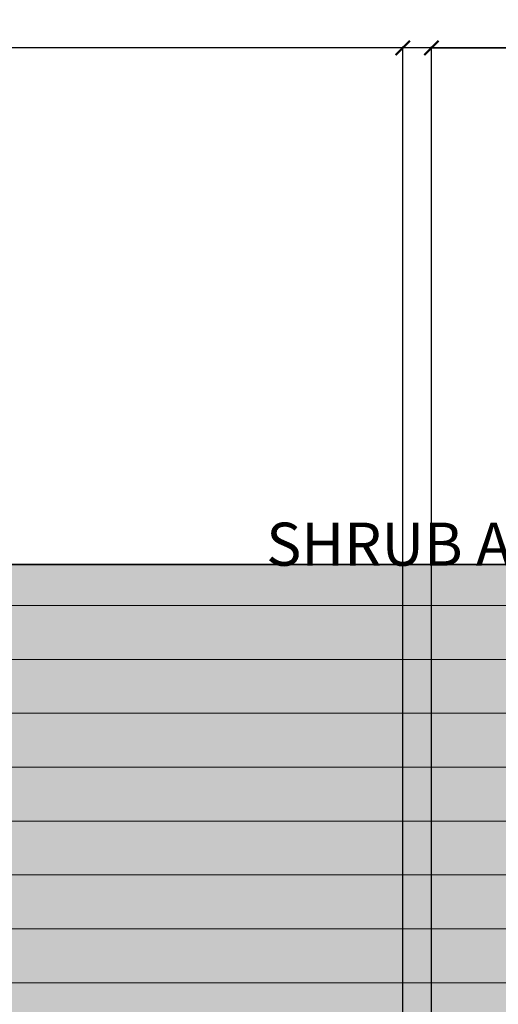
# Model space of a CAD drawing. Units: inches. Extents: x 1704 to 6393, y -157 to 1172.
# Tile 97 of 122: x 2494 to 2561, y 972 to 1109. Entities that reach past the tile are written whole.
import ezdxf

# ---------------------------------------------------------------- set-up
doc = ezdxf.new("R2010")
doc.units = ezdxf.units.IN
doc.header["$MEASUREMENT"] = 0
for name, color, linetype, lineweight in [('A-ANNO-DIMS', 7, 'Continuous', 13), ('C-PROP', 7, 'Continuous', 35), ('L-DECK-PLNK-PATT', 250, 'Continuous', 13)]:
    doc.layers.add(name, color=color, linetype=linetype, lineweight=lineweight)
doc.layers.add('L-DECK-PATT', color=35, linetype='Continuous', lineweight=13, true_color=0xa6725b)
doc.styles.get("Standard").update_dxf_attribs({"font": 'arial.ttf'})
doc.dimstyles.get("Standard").update_dxf_attribs({"dimtxt": 6, "dimasz": 2, "dimexe": 0.18, "dimexo": 0.0625, "dimgap": 0.09, "dimtad": 0, "dimtih": 1, "dimtoh": 1, "dimdec": 1, "dimzin": 0, "dimdsep": 46, "dimlunit": 3, "dimtxsty": 'Standard', "dimblk": 'ARCHTICK', "dimcen": 0.09, "dimadec": 0, "dimazin": 0, "dimtfac": 1, "dimtdec": 1, "dimtofl": 0, "dimtmove": 0, "dimatfit": 3, "dimfxl": 1, "dimtolj": 1, "dimtzin": 0, "dimarcsym": 0})

# ---------------------------------------------------------------- blocks, each defined once
blk = doc.blocks.new('_ArchTick')
at = {"color": 0, "linetype": 'ByBlock', "const_width": 0.15}
blk.add_lwpolyline([(-0.5, -0.5), (0.5, 0.5)], dxfattribs=at)
blk = doc.blocks.new('*D88')
at = {"layer": 'A-ANNO-DIMS', "color": 0, "lineweight": -2, "transparency": 16777216}
for p, q in [((2596.64, 1031.77), (2596.64, 1036.22)), ((2625.54, 1031.77), (2625.54, 1036.22)), ((2596.64, 1036.04), (2594.64, 1036.04)), ((2625.54, 1036.04), (2596.64, 1036.04))]:
    blk.add_line(p, q, dxfattribs=at)
at = {"layer": 'Defpoints', "color": 0, "lineweight": -3, "transparency": 16777216}
for p in [(2596.64, 1036.04), (2596.64, 1031.71), (2625.54, 1031.71)]:
    blk.add_point(p, dxfattribs=at)
at = {"layer": 'A-ANNO-DIMS', "color": 0, "lineweight": -2, "transparency": 16777216, "xscale": 2, "yscale": 2, "zscale": 2, "rotation": 180}
blk.add_blockref('_ArchTick', (2596.64, 1036.04), dxfattribs=at)
at = {"layer": 'A-ANNO-DIMS', "color": 0, "lineweight": -2, "transparency": 16777216, "xscale": 2, "yscale": 2, "zscale": 2}
blk.add_blockref('_ArchTick', (2625.54, 1036.04), dxfattribs=at)
at = {"layer": 'A-ANNO-DIMS', "color": 0, "transparency": 16777216, "insert": (2560.17, 1036.04), "char_height": 6, "attachment_point": 5}
blk.add_mtext('\\A1;SHRUB A 29 TYP.', dxfattribs=at)
blk = doc.blocks.new('*D92')
at = {"layer": 'A-ANNO-DIMS', "color": 0, "lineweight": -2, "transparency": 16777216}
for p, q in [((2073.35, 895.28), (2073.35, 1105.29)), ((2073.35, 1105.11), (2332.66, 1105.11)), ((2605.35, 1105.11), (2346.04, 1105.11)), ((2605.35, 895.28), (2605.35, 1105.29))]:
    blk.add_line(p, q, dxfattribs=at)
at = {"layer": 'Defpoints', "color": 0, "lineweight": -3, "transparency": 16777216}
for p in [(2605.35, 1105.11), (2073.35, 895.21), (2605.35, 895.21)]:
    blk.add_point(p, dxfattribs=at)
at = {"layer": 'A-ANNO-DIMS', "color": 0, "lineweight": -2, "transparency": 16777216, "xscale": 2, "yscale": 2, "zscale": 2, "rotation": 180}
blk.add_blockref('_ArchTick', (2073.35, 1105.11), dxfattribs=at)
at = {"layer": 'A-ANNO-DIMS', "color": 0, "lineweight": -2, "transparency": 16777216, "xscale": 2, "yscale": 2, "zscale": 2}
blk.add_blockref('_ArchTick', (2605.35, 1105.11), dxfattribs=at)
at = {"layer": 'A-ANNO-DIMS', "color": 0, "transparency": 16777216, "insert": (2339.35, 1105.11), "char_height": 6, "attachment_point": 5}
blk.add_mtext('\\A1;532', dxfattribs=at)
blk = doc.blocks.new('*D102')
at = {"layer": 'A-ANNO-DIMS', "color": 0, "lineweight": -2, "transparency": 16777216}
for p, q in [((2367.74, 711.28), (2367.74, 1105.29)), ((2367.74, 1105.11), (2447.61, 1105.11)), ((2547.35, 1105.11), (2467.47, 1105.11)), ((2547.35, 711.28), (2547.35, 1105.29))]:
    blk.add_line(p, q, dxfattribs=at)
at = {"layer": 'Defpoints', "color": 0, "lineweight": -3, "transparency": 16777216}
for p in [(2547.35, 1105.11), (2367.74, 711.21), (2547.35, 711.21)]:
    blk.add_point(p, dxfattribs=at)
at = {"layer": 'A-ANNO-DIMS', "color": 0, "lineweight": -2, "transparency": 16777216, "xscale": 2, "yscale": 2, "zscale": 2, "rotation": 180}
blk.add_blockref('_ArchTick', (2367.74, 1105.11), dxfattribs=at)
at = {"layer": 'A-ANNO-DIMS', "color": 0, "lineweight": -2, "transparency": 16777216, "xscale": 2, "yscale": 2, "zscale": 2}
blk.add_blockref('_ArchTick', (2547.35, 1105.11), dxfattribs=at)
at = {"layer": 'A-ANNO-DIMS', "color": 0, "transparency": 16777216, "insert": (2457.54, 1105.11), "char_height": 6, "attachment_point": 5}
blk.add_mtext('\\A1;179.6', dxfattribs=at)
blk = doc.blocks.new('*D103')
at = {"layer": 'A-ANNO-DIMS', "color": 0, "lineweight": -2, "transparency": 16777216}
for p, q in [((2551.35, 711.28), (2551.35, 1105.29)), ((2551.35, 1105.11), (2569.84, 1105.11)), ((2597.35, 1105.11), (2578.85, 1105.11)), ((2597.35, 711.28), (2597.35, 1105.29))]:
    blk.add_line(p, q, dxfattribs=at)
at = {"layer": 'Defpoints', "color": 0, "lineweight": -3, "transparency": 16777216}
for p in [(2597.35, 1105.11), (2551.35, 711.21), (2597.35, 711.21)]:
    blk.add_point(p, dxfattribs=at)
at = {"layer": 'A-ANNO-DIMS', "color": 0, "lineweight": -2, "transparency": 16777216, "xscale": 2, "yscale": 2, "zscale": 2, "rotation": 180}
blk.add_blockref('_ArchTick', (2551.35, 1105.11), dxfattribs=at)
at = {"layer": 'A-ANNO-DIMS', "color": 0, "lineweight": -2, "transparency": 16777216, "xscale": 2, "yscale": 2, "zscale": 2}
blk.add_blockref('_ArchTick', (2597.35, 1105.11), dxfattribs=at)
at = {"layer": 'A-ANNO-DIMS', "color": 0, "transparency": 16777216, "insert": (2574.35, 1105.11), "char_height": 6, "attachment_point": 5}
blk.add_mtext('\\A1;46', dxfattribs=at)

msp = doc.modelspace()

# ---------------------------------------------------------------- hatches: boundary and pattern name
at = {"layer": 'L-DECK-PATT', "transparency": 33554544}
h = msp.add_hatch(color=256, dxfattribs=at)
h.dxf.hatch_style = 1
h.paths.add_polyline_path([(2329.589, 1033.213), (2065.589, 1033.213), (2065.589, 895.213), (2167.349, 895.213), (2263.349, 895.213), (2263.349, 903.213), (2273.349, 903.213), (2273.349, 895.213), (2329.589, 895.213)])
h.paths.add_polyline_path([(2664.349, 1033.213), (2333.589, 1033.213), (2333.589, 895.213), (2465.349, 895.213), (2469.181, 895.213), (2470.482, 895.213), (2508.215, 895.213), (2509.516, 895.213), (2513.349, 895.213), (2533.349, 895.213), (2581.349, 895.213), (2605.349, 895.213), (2664.349, 895.213)])
h.paths.add_polyline_path([(2333.589, 1033.213), (2329.589, 1033.213), (2329.589, 895.213), (2333.589, 895.213)])
at = {"layer": 'L-DECK-PLNK-PATT'}
h = msp.add_hatch(dxfattribs=at)
h.set_pattern_fill('LINE', color=256, scale=60)
h.paths.add_polyline_path([(2329.589, 1033.213), (2065.589, 1033.213), (2065.589, 895.213), (2167.349, 895.213), (2263.349, 895.213), (2263.349, 903.213), (2273.349, 903.213), (2273.349, 895.213), (2329.589, 895.213)])
h.paths.add_polyline_path([(2664.349, 1033.213), (2333.589, 1033.213), (2333.589, 895.213), (2465.349, 895.213), (2469.181, 895.213), (2470.482, 895.213), (2508.215, 895.213), (2509.516, 895.213), (2513.349, 895.213), (2533.349, 895.213), (2581.349, 895.213), (2605.349, 895.213), (2664.349, 895.213)])
h.paths.add_polyline_path([(2333.589, 1033.213), (2329.589, 1033.213), (2329.589, 895.213), (2333.589, 895.213)])

# ---------------------------------------------------------------- linework, layer by layer
at = {"layer": 'C-PROP'}
msp.add_line((2723.349, 1033.213), (1898.349, 1033.213), dxfattribs=at)

# ---------------------------------------------------------------- dimensions: what is measured, and where the dimension line sits
at = {"layer": 'A-ANNO-DIMS'}
for base, p1, p2, override, picture, middle in [((2605.349, 1105.107), (2073.349, 895.213), (2605.349, 895.213), {"dimdec": 0, "dimlfac": 1, "dimrnd": 0, "dimzin": 0, "dimdsep": 46, "dimlunit": 2}, '*D92', (2339.349, 1105.107)), ((2547.349, 1105.107), (2367.738, 711.213), (2547.349, 711.213), {"dimdec": 1, "dimlfac": 1, "dimrnd": 0, "dimzin": 0, "dimdsep": 46, "dimlunit": 2}, '*D102', (2457.543, 1105.107)), ((2597.349, 1105.107), (2551.349, 711.213), (2597.349, 711.213), {"dimdec": 0, "dimlfac": 1, "dimrnd": 0, "dimzin": 0, "dimdsep": 46, "dimlunit": 2}, '*D103', (2574.349, 1105.107))]:
    dim = msp.add_linear_dim(base=base, p1=p1, p2=p2, dimstyle='Standard', override=override, dxfattribs=at)
    dim.commit()
    dim.dimension.update_dxf_attribs({"geometry": picture, "text_midpoint": middle})
dim = msp.add_linear_dim(base=(2596.639, 1036.042), p1=(2625.54, 1031.707), p2=(2596.639, 1031.707), angle=180, text='SHRUB A <> TYP.', dimstyle='Standard', override={"dimdec": 0, "dimlfac": 1, "dimrnd": 0, "dimzin": 0, "dimdsep": 46, "dimlunit": 2}, dxfattribs=at)
dim.commit()
dim.dimension.update_dxf_attribs({"geometry": '*D88', "text_midpoint": (2560.165, 1036.042)})

doc.saveas('drawing.dxf')
